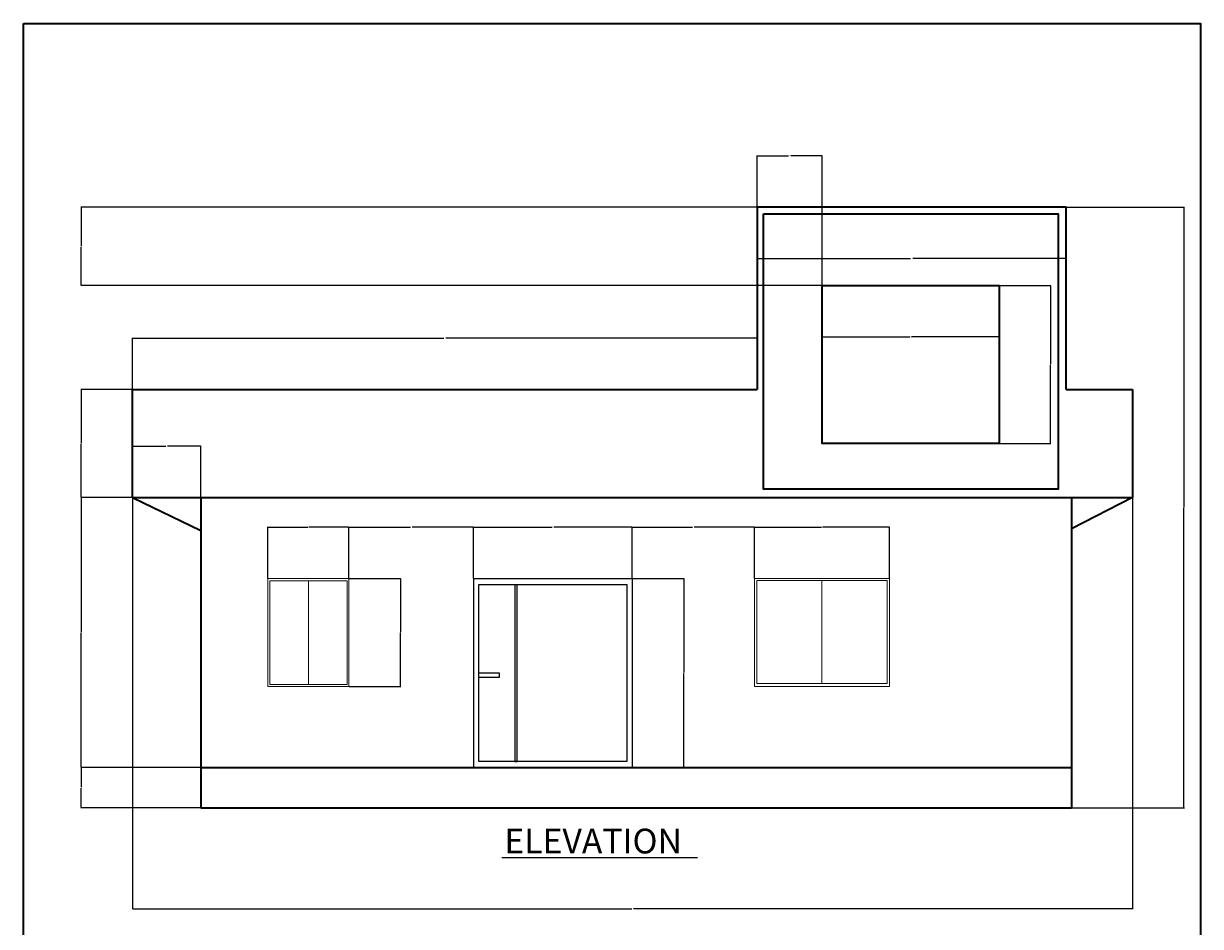
# Model space of a CAD drawing. Units: inches. Extents: x 1676 to 2199, y 1657 to 2783.
# Tile 10 of 10: x 1676 to 2199, y 2381 to 2783. Entities that reach past the tile are written whole.
import ezdxf

# ---------------------------------------------------------------- set-up
doc = ezdxf.new("R2010")
doc.units = ezdxf.units.IN
for name, color, linetype, lineweight in [('A-ANNO-DIMS', 2, 'Continuous', 18), ('A-ANNO-TEXT', 7, 'Continuous', 25), ('A-ANNO-TTLB', 7, 'Continuous', 35), ('A-ELEV', 7, 'Continuous', 35), ('A-ELEV-DOOR', 4, 'Continuous', 25), ('A-ELEV-GLAZ', 4, 'Continuous', 18)]:
    doc.layers.add(name, color=color, linetype=linetype, lineweight=lineweight)
doc.styles.get("Standard").update_dxf_attribs({"font": 'arial.ttf'})
doc.dimstyles.get("Standard").update_dxf_attribs({"dimtxt": 0.18, "dimasz": 0.18, "dimexe": 0.18, "dimexo": 0.0625, "dimgap": 0.09, "dimtad": 0, "dimtih": 1, "dimtoh": 1, "dimdec": 4, "dimzin": 0, "dimdsep": 46, "dimtxsty": 'Standard', "dimcen": 0.09, "dimadec": 0, "dimazin": 0, "dimtfac": 1, "dimtdec": 4, "dimtofl": 0, "dimtmove": 0, "dimatfit": 3, "dimfxl": 1, "dimtolj": 1, "dimtzin": 0, "dimarcsym": 0})

# ---------------------------------------------------------------- blocks, each defined once
blk = doc.blocks.new('*D59')
at = {"layer": 'A-ANNO-DIMS', "color": 0, "lineweight": -2, "transparency": 16777216}
for p, q in [((1724.76, 2571.7), (1724.76, 2388.72)), ((2169.27, 2571.7), (2169.27, 2388.72)), ((1724.94, 2388.9), (1946.62, 2388.9)), ((2169.09, 2388.9), (1947.42, 2388.9))]:
    blk.add_line(p, q, dxfattribs=at)
at = {"layer": 'A-ANNO-DIMS', "color": 0, "transparency": 16777216}
for points in [[(1724.94, 2388.93), (1724.94, 2388.87), (1724.76, 2388.9)], [(2169.09, 2388.93), (2169.09, 2388.87), (2169.27, 2388.9)]]:
    blk.add_solid(points, dxfattribs=at)
at = {"layer": 'Defpoints', "color": 0, "transparency": 16777216}
for p in [(1724.76, 2571.76), (2169.27, 2571.76), (2169.27, 2388.9)]:
    blk.add_point(p, dxfattribs=at)
at = {"layer": 'A-ANNO-DIMS', "color": 0, "transparency": 16777216, "insert": (1947.02, 2388.9), "char_height": 0.18, "attachment_point": 5}
blk.add_mtext('\\A1;444.5', dxfattribs=at)
blk = doc.blocks.new('*D60')
at = {"layer": 'A-ANNO-DIMS', "color": 0, "lineweight": -2, "transparency": 16777216}
for p, q in [((1724.76, 2619.82), (1724.76, 2642.79)), ((1724.94, 2642.61), (1863.12, 2642.61)), ((2002.23, 2642.61), (1864.05, 2642.61)), ((2002.41, 2619.82), (2002.41, 2642.79))]:
    blk.add_line(p, q, dxfattribs=at)
at = {"layer": 'A-ANNO-DIMS', "color": 0, "transparency": 16777216}
for points in [[(1724.94, 2642.64), (1724.94, 2642.58), (1724.76, 2642.61)], [(2002.23, 2642.64), (2002.23, 2642.58), (2002.41, 2642.61)]]:
    blk.add_solid(points, dxfattribs=at)
at = {"layer": 'Defpoints', "color": 0, "transparency": 16777216}
for p in [(2002.41, 2642.61), (1724.76, 2619.76), (2002.41, 2619.76)]:
    blk.add_point(p, dxfattribs=at)
at = {"layer": 'A-ANNO-DIMS', "color": 0, "transparency": 16777216, "insert": (1863.59, 2642.61), "char_height": 0.18, "attachment_point": 5}
blk.add_mtext('\\A1;277.65', dxfattribs=at)
blk = doc.blocks.new('*D61')
at = {"layer": 'A-ANNO-DIMS', "color": 0, "lineweight": -2, "transparency": 16777216}
for p, q in [((2002.41, 2700.81), (2002.41, 2677.84)), ((2139.74, 2700.81), (2139.74, 2677.84)), ((2002.59, 2678.02), (2070.62, 2678.02)), ((2139.56, 2678.02), (2071.53, 2678.02))]:
    blk.add_line(p, q, dxfattribs=at)
at = {"layer": 'A-ANNO-DIMS', "color": 0, "transparency": 16777216}
for points in [[(2002.59, 2678.05), (2002.59, 2677.99), (2002.41, 2678.02)], [(2139.56, 2678.05), (2139.56, 2677.99), (2139.74, 2678.02)]]:
    blk.add_solid(points, dxfattribs=at)
at = {"layer": 'Defpoints', "color": 0, "transparency": 16777216}
for p in [(2002.41, 2700.87), (2139.74, 2700.87), (2002.41, 2678.02)]:
    blk.add_point(p, dxfattribs=at)
at = {"layer": 'A-ANNO-DIMS', "color": 0, "transparency": 16777216, "insert": (2071.08, 2678.02), "char_height": 0.18, "attachment_point": 5}
blk.add_mtext('\\A1;137.33', dxfattribs=at)
blk = doc.blocks.new('*D62')
at = {"layer": 'A-ANNO-DIMS', "color": 0, "lineweight": -2, "transparency": 16777216}
for p, q in [((2031.26, 2665.93), (2031.26, 2642.97)), ((2109.97, 2665.93), (2109.97, 2642.97)), ((2031.44, 2643.15), (2070.22, 2643.15)), ((2109.79, 2643.15), (2071.01, 2643.15))]:
    blk.add_line(p, q, dxfattribs=at)
at = {"layer": 'A-ANNO-DIMS', "color": 0, "transparency": 16777216}
for points in [[(2031.44, 2643.18), (2031.44, 2643.12), (2031.26, 2643.15)], [(2109.79, 2643.18), (2109.79, 2643.12), (2109.97, 2643.15)]]:
    blk.add_solid(points, dxfattribs=at)
at = {"layer": 'Defpoints', "color": 0, "transparency": 16777216}
for p in [(2031.26, 2666), (2109.97, 2666), (2031.26, 2643.15)]:
    blk.add_point(p, dxfattribs=at)
at = {"layer": 'A-ANNO-DIMS', "color": 0, "transparency": 16777216, "insert": (2070.61, 2643.15), "char_height": 0.18, "attachment_point": 5}
blk.add_mtext('\\A1;78.72', dxfattribs=at)
blk = doc.blocks.new('*D63')
at = {"layer": 'A-ANNO-DIMS', "color": 0, "lineweight": -2, "transparency": 16777216}
for p, q in [((2110.03, 2666), (2133, 2666)), ((2132.82, 2665.82), (2132.82, 2631.07)), ((2132.82, 2595.97), (2132.82, 2630.71)), ((2110.03, 2595.79), (2133, 2595.79))]:
    blk.add_line(p, q, dxfattribs=at)
at = {"layer": 'A-ANNO-DIMS', "color": 0, "transparency": 16777216}
for points in [[(2132.79, 2665.82), (2132.85, 2665.82), (2132.82, 2666)], [(2132.79, 2595.97), (2132.85, 2595.97), (2132.82, 2595.79)]]:
    blk.add_solid(points, dxfattribs=at)
at = {"layer": 'Defpoints', "color": 0, "transparency": 16777216}
for p in [(2109.97, 2666), (2109.97, 2595.79), (2132.82, 2595.79)]:
    blk.add_point(p, dxfattribs=at)
at = {"layer": 'A-ANNO-DIMS', "color": 0, "transparency": 16777216, "insert": (2132.82, 2630.89), "char_height": 0.18, "attachment_point": 5}
blk.add_mtext('\\A1;70.21', dxfattribs=at)
blk = doc.blocks.new('*D64')
at = {"layer": 'A-ANNO-DIMS', "color": 0, "lineweight": -2, "transparency": 16777216}
for p, q in [((2002.41, 2700.94), (2002.41, 2723.9)), ((2002.59, 2723.72), (2016.37, 2723.72)), ((2031.08, 2723.72), (2017.3, 2723.72)), ((2031.26, 2666.06), (2031.26, 2723.9))]:
    blk.add_line(p, q, dxfattribs=at)
at = {"layer": 'A-ANNO-DIMS', "color": 0, "transparency": 16777216}
for points in [[(2002.59, 2723.75), (2002.59, 2723.69), (2002.41, 2723.72)], [(2031.08, 2723.75), (2031.08, 2723.69), (2031.26, 2723.72)]]:
    blk.add_solid(points, dxfattribs=at)
at = {"layer": 'Defpoints', "color": 0, "transparency": 16777216}
for p in [(2002.41, 2723.72), (2002.41, 2700.87), (2031.26, 2666)]:
    blk.add_point(p, dxfattribs=at)
at = {"layer": 'A-ANNO-DIMS', "color": 0, "transparency": 16777216, "insert": (2016.83, 2723.72), "char_height": 0.18, "attachment_point": 5}
blk.add_mtext('\\A1;28.843', dxfattribs=at)
blk = doc.blocks.new('*D65')
at = {"layer": 'A-ANNO-DIMS', "color": 0, "lineweight": -2, "transparency": 16777216}
for p, q in [((2002.35, 2700.87), (1701.73, 2700.87)), ((1701.91, 2700.69), (1701.91, 2683.62)), ((1701.91, 2666.18), (1701.91, 2683.25)), ((2031.19, 2666), (1701.73, 2666))]:
    blk.add_line(p, q, dxfattribs=at)
at = {"layer": 'A-ANNO-DIMS', "color": 0, "transparency": 16777216}
for points in [[(1701.88, 2700.69), (1701.94, 2700.69), (1701.91, 2700.87)], [(1701.88, 2666.18), (1701.94, 2666.18), (1701.91, 2666)]]:
    blk.add_solid(points, dxfattribs=at)
at = {"layer": 'Defpoints', "color": 0, "transparency": 16777216}
for p in [(1701.91, 2700.87), (2002.41, 2700.87), (2031.26, 2666)]:
    blk.add_point(p, dxfattribs=at)
at = {"layer": 'A-ANNO-DIMS', "color": 0, "transparency": 16777216, "insert": (1701.91, 2683.44), "char_height": 0.18, "attachment_point": 5}
blk.add_mtext('\\A1;34.88', dxfattribs=at)
blk = doc.blocks.new('*D66')
at = {"layer": 'A-ANNO-DIMS', "color": 0, "lineweight": -2, "transparency": 16777216}
for p, q in [((2139.81, 2700.87), (2192.3, 2700.87)), ((2192.12, 2700.69), (2192.12, 2567.5)), ((2192.12, 2433.94), (2192.12, 2567.14)), ((2142.14, 2433.76), (2192.3, 2433.76))]:
    blk.add_line(p, q, dxfattribs=at)
at = {"layer": 'A-ANNO-DIMS', "color": 0, "transparency": 16777216}
for points in [[(2192.09, 2700.69), (2192.15, 2700.69), (2192.12, 2700.87)], [(2192.09, 2433.94), (2192.15, 2433.94), (2192.12, 2433.76)]]:
    blk.add_solid(points, dxfattribs=at)
at = {"layer": 'Defpoints', "color": 0, "transparency": 16777216}
for p in [(2139.74, 2700.87), (2192.12, 2700.87), (2142.07, 2433.76)]:
    blk.add_point(p, dxfattribs=at)
at = {"layer": 'A-ANNO-DIMS', "color": 0, "transparency": 16777216, "insert": (2192.12, 2567.32), "char_height": 0.18, "attachment_point": 5}
blk.add_mtext('\\A1;267.1', dxfattribs=at)
blk = doc.blocks.new('*D67')
at = {"layer": 'A-ANNO-DIMS', "color": 0, "lineweight": -2, "transparency": 16777216}
for p, q in [((1755.01, 2451.76), (1701.73, 2451.76)), ((1701.91, 2451.58), (1701.91, 2442.94)), ((1701.91, 2433.94), (1701.91, 2442.58)), ((1755.01, 2433.76), (1701.73, 2433.76))]:
    blk.add_line(p, q, dxfattribs=at)
at = {"layer": 'A-ANNO-DIMS', "color": 0, "transparency": 16777216}
for points in [[(1701.88, 2451.58), (1701.94, 2451.58), (1701.91, 2451.76)], [(1701.88, 2433.94), (1701.94, 2433.94), (1701.91, 2433.76)]]:
    blk.add_solid(points, dxfattribs=at)
at = {"layer": 'Defpoints', "color": 0, "transparency": 16777216}
for p in [(1701.91, 2451.76), (1755.07, 2451.76), (1755.07, 2433.76)]:
    blk.add_point(p, dxfattribs=at)
at = {"layer": 'A-ANNO-DIMS', "color": 0, "transparency": 16777216, "insert": (1701.91, 2442.76), "char_height": 0.18, "attachment_point": 5}
blk.add_mtext('\\A1;18', dxfattribs=at)
blk = doc.blocks.new('*D68')
at = {"layer": 'A-ANNO-DIMS', "color": 0, "lineweight": -2, "transparency": 16777216}
for p, q in [((1755.01, 2571.76), (1701.73, 2571.76)), ((1701.91, 2571.58), (1701.91, 2511.94)), ((1701.91, 2451.94), (1701.91, 2511.58)), ((1755.01, 2451.76), (1701.73, 2451.76))]:
    blk.add_line(p, q, dxfattribs=at)
at = {"layer": 'A-ANNO-DIMS', "color": 0, "transparency": 16777216}
for points in [[(1701.88, 2571.58), (1701.94, 2571.58), (1701.91, 2571.76)], [(1701.88, 2451.94), (1701.94, 2451.94), (1701.91, 2451.76)]]:
    blk.add_solid(points, dxfattribs=at)
at = {"layer": 'Defpoints', "color": 0, "transparency": 16777216}
for p in [(1701.91, 2571.76), (1755.07, 2571.76), (1755.07, 2451.76)]:
    blk.add_point(p, dxfattribs=at)
at = {"layer": 'A-ANNO-DIMS', "color": 0, "transparency": 16777216, "insert": (1701.91, 2511.76), "char_height": 0.18, "attachment_point": 5}
blk.add_mtext('\\A1;120', dxfattribs=at)
blk = doc.blocks.new('*D69')
at = {"layer": 'A-ANNO-DIMS', "color": 0, "lineweight": -2, "transparency": 16777216}
for p, q in [((1820.99, 2535.76), (1843.95, 2535.76)), ((1843.77, 2535.58), (1843.77, 2511.94)), ((1843.77, 2487.94), (1843.77, 2511.58)), ((1820.99, 2487.76), (1843.95, 2487.76))]:
    blk.add_line(p, q, dxfattribs=at)
at = {"layer": 'A-ANNO-DIMS', "color": 0, "transparency": 16777216}
for points in [[(1843.74, 2535.58), (1843.8, 2535.58), (1843.77, 2535.76)], [(1843.74, 2487.94), (1843.8, 2487.94), (1843.77, 2487.76)]]:
    blk.add_solid(points, dxfattribs=at)
at = {"layer": 'Defpoints', "color": 0, "transparency": 16777216}
for p in [(1820.92, 2535.76), (1820.92, 2487.76), (1843.77, 2487.76)]:
    blk.add_point(p, dxfattribs=at)
at = {"layer": 'A-ANNO-DIMS', "color": 0, "transparency": 16777216, "insert": (1843.77, 2511.76), "char_height": 0.18, "attachment_point": 5}
blk.add_mtext('\\A1;48', dxfattribs=at)
blk = doc.blocks.new('*D70')
at = {"layer": 'A-ANNO-DIMS', "color": 0, "lineweight": -2, "transparency": 16777216}
for p, q in [((1946.94, 2535.76), (1969.91, 2535.76)), ((1969.73, 2535.58), (1969.73, 2493.94)), ((1969.73, 2451.94), (1969.73, 2493.58)), ((1946.94, 2451.76), (1969.91, 2451.76))]:
    blk.add_line(p, q, dxfattribs=at)
at = {"layer": 'A-ANNO-DIMS', "color": 0, "transparency": 16777216}
for points in [[(1969.7, 2535.58), (1969.76, 2535.58), (1969.73, 2535.76)], [(1969.7, 2451.94), (1969.76, 2451.94), (1969.73, 2451.76)]]:
    blk.add_solid(points, dxfattribs=at)
at = {"layer": 'Defpoints', "color": 0, "transparency": 16777216}
for p in [(1946.88, 2535.76), (1946.88, 2451.76), (1969.73, 2451.76)]:
    blk.add_point(p, dxfattribs=at)
at = {"layer": 'A-ANNO-DIMS', "color": 0, "transparency": 16777216, "insert": (1969.73, 2493.76), "char_height": 0.18, "attachment_point": 5}
blk.add_mtext('\\A1;84', dxfattribs=at)
blk = doc.blocks.new('*D71')
at = {"layer": 'A-ANNO-DIMS', "color": 0, "lineweight": -2, "transparency": 16777216}
for p, q in [((1724.7, 2619.76), (1701.73, 2619.76)), ((1701.91, 2619.58), (1701.91, 2595.94)), ((1701.91, 2571.94), (1701.91, 2595.58)), ((1724.7, 2571.76), (1701.73, 2571.76))]:
    blk.add_line(p, q, dxfattribs=at)
at = {"layer": 'A-ANNO-DIMS', "color": 0, "transparency": 16777216}
for points in [[(1701.88, 2619.58), (1701.94, 2619.58), (1701.91, 2619.76)], [(1701.88, 2571.94), (1701.94, 2571.94), (1701.91, 2571.76)]]:
    blk.add_solid(points, dxfattribs=at)
at = {"layer": 'Defpoints', "color": 0, "transparency": 16777216}
for p in [(1701.91, 2619.76), (1724.76, 2619.76), (1724.76, 2571.76)]:
    blk.add_point(p, dxfattribs=at)
at = {"layer": 'A-ANNO-DIMS', "color": 0, "transparency": 16777216, "insert": (1701.91, 2595.76), "char_height": 0.18, "attachment_point": 5}
blk.add_mtext('\\A1;48', dxfattribs=at)
blk = doc.blocks.new('*D72')
at = {"layer": 'A-ANNO-DIMS', "color": 0, "lineweight": -2, "transparency": 16777216}
for p, q in [((1784.92, 2535.82), (1784.92, 2558.79)), ((1785.1, 2558.61), (1802.7, 2558.61)), ((1820.74, 2558.61), (1803.14, 2558.61)), ((1820.92, 2535.82), (1820.92, 2558.79))]:
    blk.add_line(p, q, dxfattribs=at)
at = {"layer": 'A-ANNO-DIMS', "color": 0, "transparency": 16777216}
for points in [[(1785.1, 2558.64), (1785.1, 2558.58), (1784.92, 2558.61)], [(1820.74, 2558.64), (1820.74, 2558.58), (1820.92, 2558.61)]]:
    blk.add_solid(points, dxfattribs=at)
at = {"layer": 'Defpoints', "color": 0, "transparency": 16777216}
for p in [(1820.92, 2558.61), (1784.92, 2535.76), (1820.92, 2535.76)]:
    blk.add_point(p, dxfattribs=at)
at = {"layer": 'A-ANNO-DIMS', "color": 0, "transparency": 16777216, "insert": (1802.92, 2558.61), "char_height": 0.18, "attachment_point": 5}
blk.add_mtext('\\A1;36', dxfattribs=at)
blk = doc.blocks.new('*D73')
at = {"layer": 'A-ANNO-DIMS', "color": 0, "lineweight": -2, "transparency": 16777216}
for p, q in [((1820.92, 2535.82), (1820.92, 2558.79)), ((1821.1, 2558.61), (1848.23, 2558.61)), ((1876.14, 2558.61), (1849.01, 2558.61)), ((1876.32, 2535.82), (1876.32, 2558.79))]:
    blk.add_line(p, q, dxfattribs=at)
at = {"layer": 'A-ANNO-DIMS', "color": 0, "transparency": 16777216}
for points in [[(1821.1, 2558.64), (1821.1, 2558.58), (1820.92, 2558.61)], [(1876.14, 2558.64), (1876.14, 2558.58), (1876.32, 2558.61)]]:
    blk.add_solid(points, dxfattribs=at)
at = {"layer": 'Defpoints', "color": 0, "transparency": 16777216}
for p in [(1876.32, 2558.61), (1820.92, 2535.76), (1876.32, 2535.76)]:
    blk.add_point(p, dxfattribs=at)
at = {"layer": 'A-ANNO-DIMS', "color": 0, "transparency": 16777216, "insert": (1848.62, 2558.61), "char_height": 0.18, "attachment_point": 5}
blk.add_mtext('\\A1;55.39', dxfattribs=at)
blk = doc.blocks.new('*D74')
at = {"layer": 'A-ANNO-DIMS', "color": 0, "lineweight": -2, "transparency": 16777216}
for p, q in [((1876.32, 2535.82), (1876.32, 2558.79)), ((1876.5, 2558.61), (1911.2, 2558.61)), ((1946.7, 2558.61), (1911.99, 2558.61)), ((1946.88, 2535.82), (1946.88, 2558.79))]:
    blk.add_line(p, q, dxfattribs=at)
at = {"layer": 'A-ANNO-DIMS', "color": 0, "transparency": 16777216}
for points in [[(1876.5, 2558.64), (1876.5, 2558.58), (1876.32, 2558.61)], [(1946.7, 2558.64), (1946.7, 2558.58), (1946.88, 2558.61)]]:
    blk.add_solid(points, dxfattribs=at)
at = {"layer": 'Defpoints', "color": 0, "transparency": 16777216}
for p in [(1946.88, 2558.61), (1876.32, 2535.76), (1946.88, 2535.76)]:
    blk.add_point(p, dxfattribs=at)
at = {"layer": 'A-ANNO-DIMS', "color": 0, "transparency": 16777216, "insert": (1911.6, 2558.61), "char_height": 0.18, "attachment_point": 5}
blk.add_mtext('\\A1;70.56', dxfattribs=at)
blk = doc.blocks.new('*D75')
at = {"layer": 'A-ANNO-DIMS', "color": 0, "lineweight": -2, "transparency": 16777216}
for p, q in [((1946.88, 2535.82), (1946.88, 2558.79)), ((1947.06, 2558.61), (1973.65, 2558.61)), ((2001.03, 2558.61), (1974.44, 2558.61)), ((2001.21, 2535.82), (2001.21, 2558.79))]:
    blk.add_line(p, q, dxfattribs=at)
at = {"layer": 'A-ANNO-DIMS', "color": 0, "transparency": 16777216}
for points in [[(1947.06, 2558.64), (1947.06, 2558.58), (1946.88, 2558.61)], [(2001.03, 2558.64), (2001.03, 2558.58), (2001.21, 2558.61)]]:
    blk.add_solid(points, dxfattribs=at)
at = {"layer": 'Defpoints', "color": 0, "transparency": 16777216}
for p in [(2001.21, 2558.61), (1946.88, 2535.76), (2001.21, 2535.76)]:
    blk.add_point(p, dxfattribs=at)
at = {"layer": 'A-ANNO-DIMS', "color": 0, "transparency": 16777216, "insert": (1974.04, 2558.61), "char_height": 0.18, "attachment_point": 5}
blk.add_mtext('\\A1;54.33', dxfattribs=at)
blk = doc.blocks.new('*D76')
at = {"layer": 'A-ANNO-DIMS', "color": 0, "lineweight": -2, "transparency": 16777216}
for p, q in [((2001.21, 2535.82), (2001.21, 2558.79)), ((2001.39, 2558.61), (2030.99, 2558.61)), ((2061.03, 2558.61), (2031.43, 2558.61)), ((2061.21, 2535.82), (2061.21, 2558.79))]:
    blk.add_line(p, q, dxfattribs=at)
at = {"layer": 'A-ANNO-DIMS', "color": 0, "transparency": 16777216}
for points in [[(2001.39, 2558.64), (2001.39, 2558.58), (2001.21, 2558.61)], [(2061.03, 2558.64), (2061.03, 2558.58), (2061.21, 2558.61)]]:
    blk.add_solid(points, dxfattribs=at)
at = {"layer": 'Defpoints', "color": 0, "transparency": 16777216}
for p in [(2061.21, 2558.61), (2001.21, 2535.76), (2061.21, 2535.76)]:
    blk.add_point(p, dxfattribs=at)
at = {"layer": 'A-ANNO-DIMS', "color": 0, "transparency": 16777216, "insert": (2031.21, 2558.61), "char_height": 0.18, "attachment_point": 5}
blk.add_mtext('\\A1;60', dxfattribs=at)
blk = doc.blocks.new('*D77')
at = {"layer": 'A-ANNO-DIMS', "color": 0, "lineweight": -2, "transparency": 16777216}
for p, q in [((1724.76, 2571.82), (1724.76, 2594.79)), ((1724.94, 2594.61), (1739.54, 2594.61)), ((1754.89, 2594.61), (1740.29, 2594.61)), ((1755.07, 2571.82), (1755.07, 2594.79))]:
    blk.add_line(p, q, dxfattribs=at)
at = {"layer": 'A-ANNO-DIMS', "color": 0, "transparency": 16777216}
for points in [[(1724.94, 2594.64), (1724.94, 2594.58), (1724.76, 2594.61)], [(1754.89, 2594.64), (1754.89, 2594.58), (1755.07, 2594.61)]]:
    blk.add_solid(points, dxfattribs=at)
at = {"layer": 'Defpoints', "color": 0, "transparency": 16777216}
for p in [(1755.07, 2594.61), (1724.76, 2571.76), (1755.07, 2571.76)]:
    blk.add_point(p, dxfattribs=at)
at = {"layer": 'A-ANNO-DIMS', "color": 0, "transparency": 16777216, "insert": (1739.92, 2594.61), "char_height": 0.18, "attachment_point": 5}
blk.add_mtext('\\A1;30.31', dxfattribs=at)

msp = doc.modelspace()

# ---------------------------------------------------------------- linework, layer by layer
at = {"layer": 'A-ANNO-TEXT'}
msp.add_line((1888.9137, 2411.7499), (1975.8773, 2411.7499), dxfattribs=at)
at = {"layer": 'A-ANNO-TTLB'}
msp.add_lwpolyline([(1676.2722, 2782.5054), (2199.4461, 2782.5054), (2199.4461, 1657.2705), (1676.2722, 1657.2705)], close=True, dxfattribs=at)
at = {"layer": 'A-ELEV'}
for p, q in [((2139.7448, 2700.8748), (2002.4134, 2700.8748)), ((2002.4134, 2700.8748), (2002.4134, 2619.7614)), ((2139.7448, 2619.7614), (2139.7448, 2700.8748)), ((1724.7621, 2619.7614), (2002.4134, 2619.7614)), ((1724.7621, 2571.7614), (1724.7621, 2619.7614)), ((2139.7448, 2619.7614), (2169.2746, 2619.7614)), ((2169.2746, 2619.7614), (2169.2746, 2571.7614)), ((1724.7621, 2571.7614), (2169.2746, 2571.7614)), ((1724.7621, 2571.7614), (1755.075, 2557.0611)), ((1755.075, 2571.7614), (1755.075, 2433.7614)), ((2142.075, 2571.7614), (2142.075, 2433.7614)), ((2169.2746, 2571.7614), (2142.075, 2557.8672)), ((1755.075, 2451.7614), (2142.075, 2451.7614)), ((1755.075, 2433.7614), (2142.075, 2433.7614))]:
    msp.add_line(p, q, dxfattribs=at)
for points in [[(2005.1965, 2697.845), (2136.2306, 2697.845), (2136.2306, 2575.4891), (2005.1965, 2575.4891)], [(2031.2564, 2665.9963), (2109.9722, 2665.9963), (2109.9722, 2595.7864), (2031.2564, 2595.7864)]]:
    msp.add_lwpolyline(points, close=True, dxfattribs=at)
at = {"layer": 'A-ELEV-DOOR'}
for p, q in [((1876.3163, 2535.7614), (1876.3163, 2451.7614)), ((1876.3163, 2535.7614), (1946.8789, 2535.7614)), ((1894.7237, 2533.1607), (1894.7237, 2454.3708)), ((1895.7237, 2454.3708), (1895.7237, 2533.1607)), ((1946.8789, 2535.7614), (1946.8789, 2451.7614)), ((1894.7237, 2454.3708), (1895.7237, 2454.3708))]:
    msp.add_line(p, q, dxfattribs=at)
for points in [[(1878.6, 2533.1607), (1944.4719, 2533.1607), (1944.4719, 2454.3708), (1878.6, 2454.3708)], [(1878.6, 2493.7657), (1887.72, 2493.7657), (1887.72, 2491.7545), (1878.6, 2491.7545)]]:
    msp.add_lwpolyline(points, close=True, dxfattribs=at)
at = {"layer": 'A-ELEV-GLAZ'}
for p, q in [((1784.9237, 2535.7614), (1820.9237, 2535.7614)), ((1784.9237, 2535.7614), (1784.9237, 2487.7614)), ((1802.9011, 2534.6604), (1802.9011, 2488.6657)), ((1820.9237, 2535.7614), (1820.9237, 2487.7614)), ((2001.2106, 2535.7614), (2001.2106, 2487.7614)), ((2001.2106, 2535.7614), (2061.2105, 2535.7614)), ((2031.1575, 2534.816), (2031.1575, 2489.1525)), ((2061.2105, 2535.7614), (2061.2105, 2487.7614)), ((1784.9237, 2487.7614), (1820.9237, 2487.7614)), ((2001.2106, 2487.7614), (2061.2105, 2487.7614))]:
    msp.add_line(p, q, dxfattribs=at)
for points in [[(1785.7077, 2534.6604), (1820.0944, 2534.6604), (1820.0944, 2488.6657), (1785.7077, 2488.6657)], [(2002.1785, 2534.816), (2060.1365, 2534.816), (2060.1365, 2489.1525), (2002.1785, 2489.1525)]]:
    msp.add_lwpolyline(points, close=True, dxfattribs=at)

# ---------------------------------------------------------------- texts
at = {"layer": 'A-ANNO-TEXT', "insert": (1890.0026, 2424.5396), "char_height": 11, "attachment_point": 1}
msp.add_mtext_dynamic_manual_height_columns('ELEVATION', width=244.812646, gutter_width=12.5, heights=[0], dxfattribs=at)

# ---------------------------------------------------------------- dimensions: what is measured, and where the dimension line sits
at = {"layer": 'A-ANNO-DIMS'}
for base, p1, p2, override, picture, middle in [((2002.4134, 2723.7248), (2031.2564, 2665.9963), (2002.4134, 2700.8748), {"dimdec": 3, "dimlfac": 1, "dimrnd": 0, "dimzin": 0, "dimdsep": 46, "dimlunit": 2}, '*D64', (2016.8349, 2723.7248)), ((1755.075, 2594.6114), (1724.7621, 2571.7614), (1755.075, 2571.7614), {"dimdec": 2, "dimlfac": 1, "dimrnd": 0, "dimzin": 0, "dimdsep": 46, "dimlunit": 2}, '*D77', (1739.9185, 2594.6114)), ((2169.2746, 2388.8999), (1724.7621, 2571.7614), (2169.2746, 2571.7614), {"dimdec": 1, "dimlfac": 1, "dimrnd": 0, "dimzin": 0, "dimdsep": 46, "dimlunit": 2}, '*D59', (1947.0183, 2388.8999)), ((1820.9237, 2558.6114), (1784.9237, 2535.7614), (1820.9237, 2535.7614), {"dimdec": 0, "dimlfac": 1, "dimrnd": 0, "dimzin": 0, "dimdsep": 46, "dimlunit": 2}, '*D72', (1802.9237, 2558.6114)), ((1876.3163, 2558.6114), (1820.9237, 2535.7614), (1876.3163, 2535.7614), {"dimdec": 2, "dimlfac": 1, "dimrnd": 0, "dimzin": 0, "dimdsep": 46, "dimlunit": 2}, '*D73', (1848.62, 2558.6114)), ((1946.8789, 2558.6114), (1876.3163, 2535.7614), (1946.8789, 2535.7614), {"dimdec": 2, "dimlfac": 1, "dimrnd": 0, "dimzin": 0, "dimdsep": 46, "dimlunit": 2}, '*D74', (1911.5976, 2558.6114)), ((2001.2106, 2558.6114), (1946.8789, 2535.7614), (2001.2106, 2535.7614), {"dimdec": 2, "dimlfac": 1, "dimrnd": 0, "dimzin": 0, "dimdsep": 46, "dimlunit": 2}, '*D75', (1974.0447, 2558.6114)), ((2061.2105, 2558.6114), (2001.2106, 2535.7614), (2061.2105, 2535.7614), {"dimdec": 0, "dimlfac": 1, "dimrnd": 0, "dimzin": 0, "dimdsep": 46, "dimlunit": 2}, '*D76', (2031.2106, 2558.6114))]:
    dim = msp.add_linear_dim(base=base, p1=p1, p2=p2, dimstyle='Standard', override=override, dxfattribs=at)
    dim.commit()
    dim.dimension.update_dxf_attribs({"geometry": picture, "text_midpoint": middle})
for base, p1, p2, angle, override, picture, middle in [((1701.9121, 2700.8748), (2031.2564, 2665.9963), (2002.4134, 2700.8748), 90, {"dimdec": 2, "dimlfac": 1, "dimrnd": 0, "dimzin": 0, "dimdsep": 46, "dimlunit": 2}, '*D65', (1701.9121, 2683.4355)), ((2002.4134, 2678.0248), (2139.7448, 2700.8748), (2002.4134, 2700.8748), 180, {"dimdec": 2, "dimlfac": 1, "dimrnd": 0, "dimzin": 0, "dimdsep": 46, "dimlunit": 2}, '*D61', (2071.0791, 2678.0248)), ((2192.1246, 2700.8748), (2142.075, 2433.7614), (2139.7448, 2700.8748), 90, {"dimdec": 1, "dimlfac": 1, "dimrnd": 0, "dimzin": 0, "dimdsep": 46, "dimlunit": 2}, '*D66', (2192.1246, 2567.3181)), ((2031.2564, 2643.1463), (2109.9722, 2665.9963), (2031.2564, 2665.9963), 180, {"dimdec": 2, "dimlfac": 1, "dimrnd": 0, "dimzin": 0, "dimdsep": 46, "dimlunit": 2}, '*D62', (2070.6143, 2643.1463)), ((2132.8222, 2595.7864), (2109.9722, 2665.9963), (2109.9722, 2595.7864), 270, {"dimdec": 2, "dimlfac": 1, "dimrnd": 0, "dimzin": 0, "dimdsep": 46, "dimlunit": 2}, '*D63', (2132.8222, 2630.8914)), ((2002.4134, 2642.6114), (1724.7621, 2619.7614), (2002.4134, 2619.7614), 0, {"dimdec": 2, "dimlfac": 1, "dimrnd": 0, "dimzin": 0, "dimdsep": 46, "dimlunit": 2}, '*D60', (1863.5877, 2642.6114)), ((1701.9121, 2619.7614), (1724.7621, 2571.7614), (1724.7621, 2619.7614), 90, {"dimdec": 0, "dimlfac": 1, "dimrnd": 0, "dimzin": 0, "dimdsep": 46, "dimlunit": 2}, '*D71', (1701.9121, 2595.7614)), ((1701.9121, 2571.7614), (1755.075, 2451.7614), (1755.075, 2571.7614), 90, {"dimdec": 0, "dimlfac": 1, "dimrnd": 0, "dimzin": 0, "dimdsep": 46, "dimlunit": 2}, '*D68', (1701.9121, 2511.7614)), ((1843.7737, 2487.7614), (1820.9237, 2535.7614), (1820.9237, 2487.7614), 270, {"dimdec": 0, "dimlfac": 1, "dimrnd": 0, "dimzin": 0, "dimdsep": 46, "dimlunit": 2}, '*D69', (1843.7737, 2511.7614)), ((1969.7289, 2451.7614), (1946.8789, 2535.7614), (1946.8789, 2451.7614), 270, {"dimdec": 0, "dimlfac": 1, "dimrnd": 0, "dimzin": 0, "dimdsep": 46, "dimlunit": 2}, '*D70', (1969.7289, 2493.7614)), ((1701.9121, 2451.7614), (1755.075, 2433.7614), (1755.075, 2451.7614), 90, {"dimdec": 0, "dimlfac": 1, "dimrnd": 0, "dimzin": 0, "dimdsep": 46, "dimlunit": 2}, '*D67', (1701.9121, 2442.7614))]:
    dim = msp.add_linear_dim(base=base, p1=p1, p2=p2, angle=angle, dimstyle='Standard', override=override, dxfattribs=at)
    dim.commit()
    dim.dimension.update_dxf_attribs({"geometry": picture, "text_midpoint": middle})

doc.saveas('drawing.dxf')
